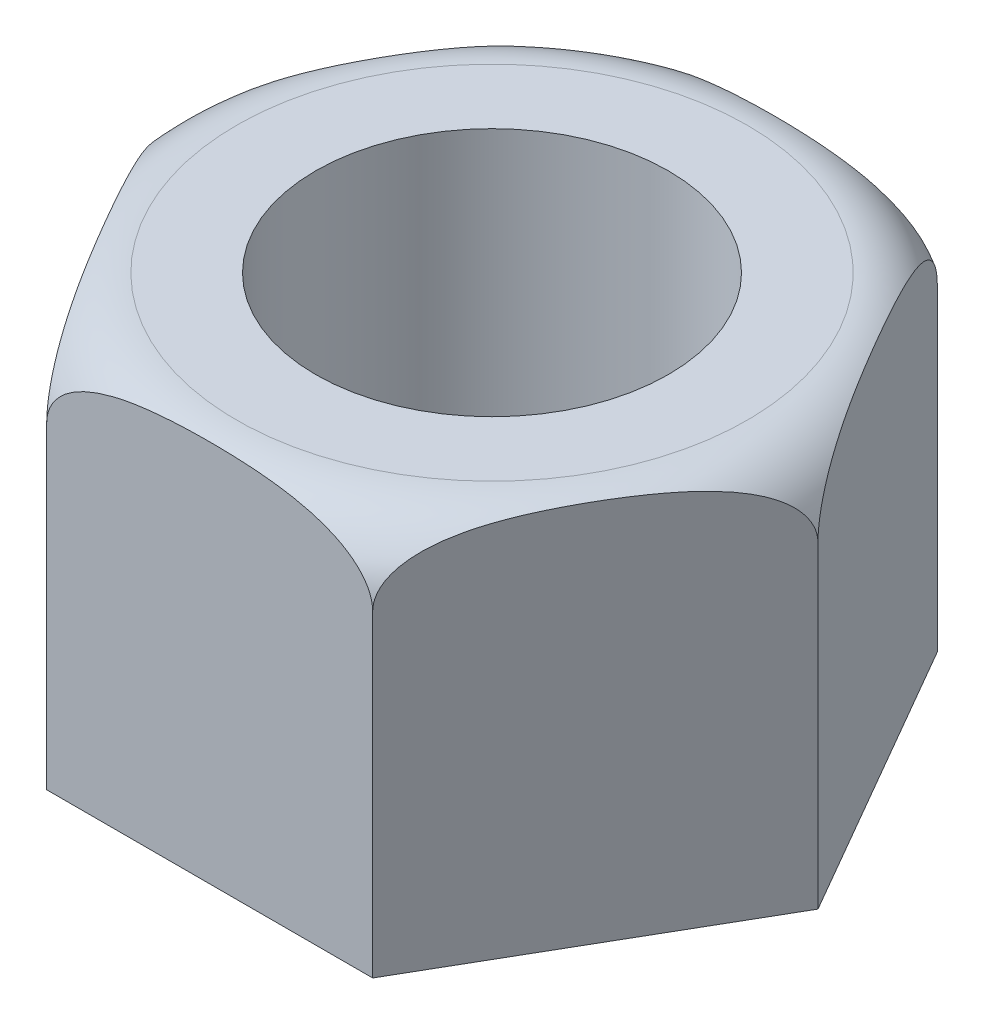
SolidWorks part; units mm, degrees
material "Plain Carbon Steel"
ref_plane "Front Plane" through (0, 0, 0) normal (0, 0, 1) x (1, 0, 0)
ref_plane "Top Plane" through (0, 0, 0) normal (0, 1, 0) x (1, 0, 0)
ref_plane "Right Plane" through (0, 0, 0) normal (1, 0, 0) x (0, 0, -1)
sketch "Hex Profile 16AF Sketch" plane through (0, 0, 0) normal (0, 1, 0) x (1, 0, 0)
  line L1 (9.2376, 0) -> (4.6188, 8)
  line L2 (4.6188, 8) -> (-4.6188, 8)
  line L3 (-4.6188, 8) -> (-9.2376, 0)
  line L4 (-9.2376, 0) -> (-4.6188, -8)
  line L5 (-4.6188, -8) -> (4.6188, -8)
  line L6 (4.6188, -8) -> (9.2376, 0)
  circle A0 centre (0, 0) radius 8 construction
  dimension "D1" = 16
extrude "Hex Body 16AF x 11" add sketch "Hex Profile 16AF Sketch" along normal mid plane 11
sketch "Chamfer Profile Sketch" plane through (0, 0, 0) normal (0, 0, 1) x (1, 0, 0)
  line L0 (9.2376, 5.5) -> (9.2376, -5.5) construction
  line L1 (4.6188, 5.5) -> (9.2376, 5.5) construction
  line L2 (9.2376, 3.5) -> (9.2376, -5.5)
  line L3 (4.6188, 5.5) -> (7.2376, 5.5)
  line L4 (0, 0) -> (0, 4.2016) construction
  line L5 (4.6188, 5.5) -> (4.6188, 7.6259)
  line L6 (4.6188, 7.6259) -> (12.103, 7.6259)
  line L7 (12.103, 7.6259) -> (12.103, -5.5)
  line L8 (12.103, -5.5) -> (9.2376, -5.5)
  arc A0 (9.2376, 3.5) -> (7.2376, 5.5) centre (7.2376, 3.5) ccw
  dimension "D1" = 2
  dimension "D2" = 12.103
  dimension "D3" = 2.1259
revolve "Face Chamfer 2mm" cut sketch "Chamfer Profile Sketch" angle 360 about L4
sketch "Bore Sketch Ø10" plane through (0, 5.5, 0) normal (0, 1, 0) x (1, 0, 0)
  circle A0 centre (0, 0) radius 5
  dimension "D1" = 10
extrude "Bore Ø10 Through" cut sketch "Bore Sketch Ø10" against normal through all
